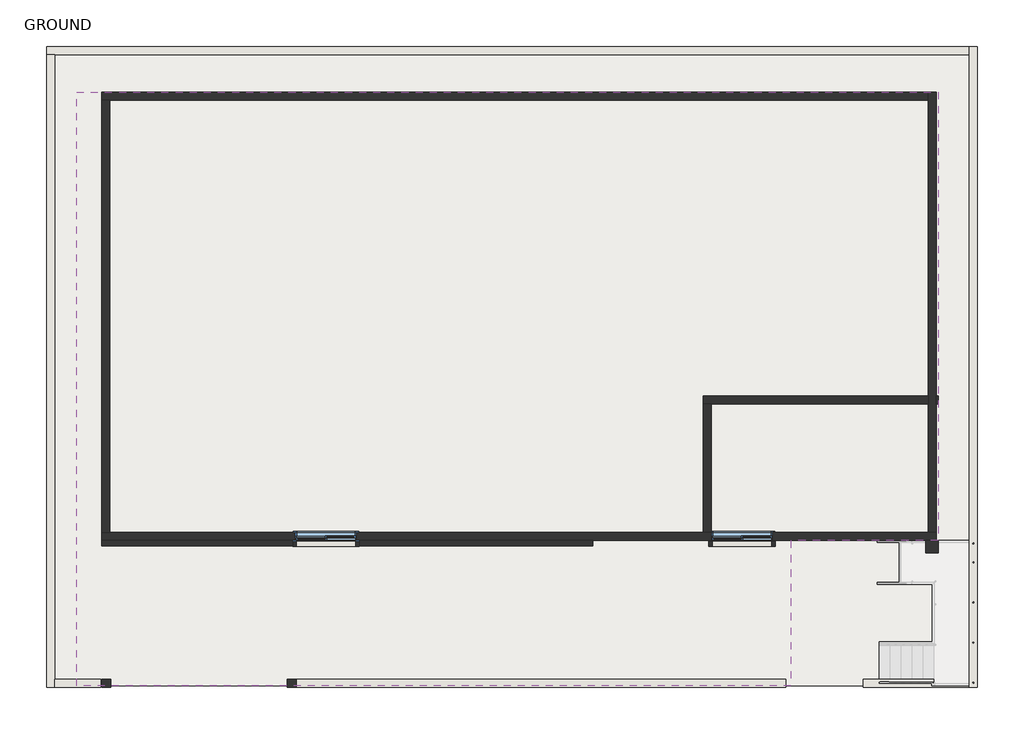
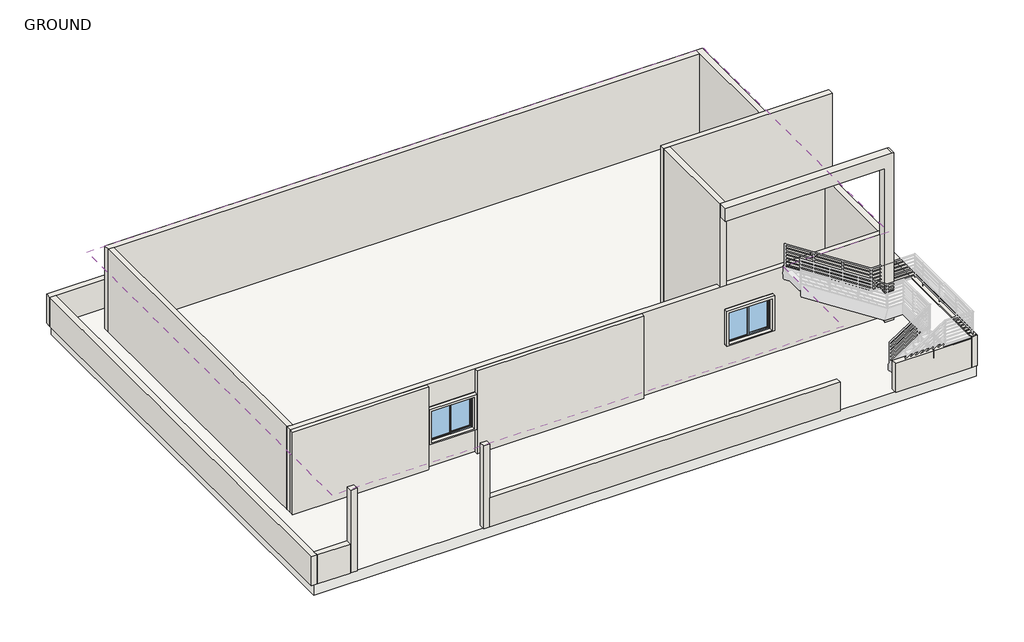
# One storey, part 1 of 4: 16 walls, 2 windows, 1 covering, 1 slab.
"""IFC4 building model written with IfcOpenShell, lengths in millimetres."""

from ifc_helpers import new_model, si_unit, frame, origin, origin_with_axes, place, context, project, spatial, polyline, outline, extrude, faceted_brep, transform, mapped, element, save
from components import walls_1_walls_1_df8d36ee, walls_2_walls_2_bd2c14ef, walls_3_walls_3_79010243, walls_4_walls_4_3dff52d5, window_c4d7a2b1

model = new_model("IFC4")

# Units and contexts
model_context = context("Model", 3, world=origin())
ifc_project = project(units=[si_unit("LENGTHUNIT", "METRE", prefix="MILLI")], contexts=[model_context])

# Site, building, storey
site = spatial("IfcSite", under=ifc_project)
building = spatial("IfcBuilding", under=site)
storey = spatial("IfcBuildingStorey", under=building, Name="GROUND", Elevation=0.0)

# Covering
placement = place(None, origin())
element("IfcCovering", 1, ObjectType="600 x 1200mm grid", at=placement, inside=storey, context=model_context, shape_type="SweptSolid", body=[
    extrude(outline(polyline([(-8160.4509113, 11210.9156744), (13293.8008502, 11210.9156744), (13293.8008502, 38.1156744), (9625.7864069, 38.1156744), (9625.7864069, -3583.7536983), (-8160.4509113, -3583.7536983), (-8160.4509113, 11210.9156744)])), frame((0.0, 0.0, 3048.0), z_axis=(0.0, 0.0, 1.0), x_axis=(1.0, 0.0, 0.0)), (0.0, 0.0, 1.0), 52.0),
])

# Slab
element("IfcSlab", 2, ObjectType="Generic Floor - 400mm", at=placement, inside=storey, context=model_context, shape_type="SweptSolid", body=[
    extrude(outline(polyline([(14250.8121881, 12248.1468238), (14250.8121881, -3583.7536983), (-8810.7878119, -3583.7536983), (-8810.7878119, 12248.1468238), (14250.8121881, 12248.1468238)])), frame((0.0, 0.0, -400.0), z_axis=(0.0, 0.0, 1.0), x_axis=(1.0, 0.0, 0.0)), (0.0, 0.0, 1.0), 400.0),
])

# Walls
element("IfcWall", 3, ObjectType="Generic - 9\"", at=placement, inside=storey, context=model_context, shape_type="Brep", body=[
    faceted_brep([(-7539.1878119, 11010.9156744, 0.0), (-7339.1878119, 11010.9156744, 0.0), (13053.0639497, 11010.9156744, 0.0), (13053.0639497, 11010.9156744, 3048.0), (-7339.1878119, 11010.9156744, 3048.0), (-7539.1878119, 11010.9156744, 3048.0), (-7539.1878119, 11210.9156744, 0.0), (-7539.1878119, 11210.9156744, 3048.0), (13053.0639497, 11210.9156744, 3048.0), (13053.0639497, 11210.9156744, 0.0)], [[[0, 1, 2, 3, 4, 5]], [[6, 7, 8, 9]], [[2, 1, 0, 6, 9]], [[5, 4, 3, 8, 7]], [[0, 5, 7, 6]], [[3, 2, 9, 8]]]),
])
element("IfcWall", 4, ObjectType="Generic - 9\"", at=placement, inside=storey, context=model_context, shape_type="SweptSolid", body=[
    extrude(outline(polyline([(-7339.1878119, 11010.9156744), (-7339.1878119, 238.1156744), (-7539.1878119, 238.1156744), (-7539.1878119, 11010.9156744), (-7339.1878119, 11010.9156744)])), origin_with_axes(), (0.0, 0.0, 1.0), 3048.0),
])
element("IfcWall", 5, ObjectType="Generic - 9\"", at=placement, inside=storey, context=model_context, shape_type="Brep", body=[
    faceted_brep([(13053.0639497, 11210.9156744, 0.0), (13053.0639497, 11010.9156744, 0.0), (13053.0639497, 3643.3156744, 0.0), (13053.0639497, 3443.3156744, 0.0), (13053.0639497, 238.1156744, 0.0), (13053.0639497, 238.1156744, 3048.0), (13053.0639497, 3443.3156744, 3048.0), (13053.0639497, 3643.3156744, 3048.0), (13053.0639497, 11010.9156744, 3048.0), (13053.0639497, 11210.9156744, 3048.0), (13253.0639497, 11210.9156744, 0.0), (13253.0639497, 11210.9156744, 3048.0), (13253.0639497, 3643.3156744, 3048.0), (13253.0639497, 3443.3156744, 3048.0), (13253.0639497, 238.1156744, 3048.0), (13253.0639497, 238.1156744, 0.0), (13253.0639497, 3443.3156744, 0.0), (13253.0639497, 3643.3156744, 0.0)], [[[0, 1, 2, 3, 4, 5, 6, 7, 8, 9]], [[10, 11, 12, 13, 14, 15, 16, 17]], [[4, 3, 2, 1, 0, 10, 17, 16, 15]], [[9, 8, 7, 6, 5, 14, 13, 12, 11]], [[0, 9, 11, 10]], [[5, 4, 15, 14]]]),
])
element("IfcWall", 6, ObjectType="Generic - 9\"", at=placement, inside=storey, context=model_context, shape_type="Brep", body=[
    faceted_brep([(-7539.1878119, 38.1156744, 0.0), (13253.0639497, 38.1156744, 0.0), (13253.0639497, 38.1156744, 3048.0), (-7539.1878119, 38.1156744, 3048.0), (-2714.7878119, 38.1156744, 2133.6), (-1190.7878119, 38.1156744, 2133.6), (-1190.7878119, 38.1156744, 914.4), (-2714.7878119, 38.1156744, 914.4), (7648.4121881, 38.1156744, 2133.6), (9172.4121881, 38.1156744, 2133.6), (9172.4121881, 38.1156744, 914.4), (7648.4121881, 38.1156744, 914.4), (-7539.1878119, 238.1156744, 0.0), (-7539.1878119, 238.1156744, 3048.0), (-7339.1878119, 238.1156744, 3048.0), (7439.6639497, 238.1156744, 3048.0), (7639.6639497, 238.1156744, 3048.0), (13053.0639497, 238.1156744, 3048.0), (13253.0639497, 238.1156744, 3048.0), (13253.0639497, 238.1156744, 0.0), (13053.0639497, 238.1156744, 0.0), (7639.6639497, 238.1156744, 0.0), (7439.6639497, 238.1156744, 0.0), (-7339.1878119, 238.1156744, 0.0), (-2714.7878119, 238.1156744, 2133.6), (-2714.7878119, 238.1156744, 914.4), (-1190.7878119, 238.1156744, 914.4), (-1190.7878119, 238.1156744, 2133.6), (7648.4121881, 238.1156744, 2133.6), (7648.4121881, 238.1156744, 914.4), (9172.4121881, 238.1156744, 914.4), (9172.4121881, 238.1156744, 2133.6)], [[[0, 1, 2, 3], [4, 5, 6, 7], [8, 9, 10, 11]], [[12, 13, 14, 15, 16, 17, 18, 19, 20, 21, 22, 23], [24, 25, 26, 27], [28, 29, 30, 31]], [[1, 0, 12, 23, 22, 21, 20, 19]], [[3, 2, 18, 17, 16, 15, 14, 13]], [[25, 24, 4, 7]], [[26, 25, 7, 6]], [[27, 26, 6, 5]], [[24, 27, 5, 4]], [[29, 28, 8, 11]], [[30, 29, 11, 10]], [[31, 30, 10, 9]], [[28, 31, 9, 8]], [[2, 1, 19, 18]], [[0, 3, 13, 12]]]),
])
element("IfcWall", 7, ObjectType="Generic - 9\"", at=placement, inside=storey, context=model_context, shape_type="Brep", body=[
    faceted_brep([(13293.8008502, 3443.3156744, 6096.0), (13093.8008502, 3443.3156744, 6096.0), (7639.6639497, 3443.3156744, 6096.0), (7439.6639497, 3443.3156744, 6096.0), (7439.6639497, 3443.3156744, 0.0), (7639.6639497, 3443.3156744, 0.0), (13053.0639497, 3443.3156744, 0.0), (13053.0639497, 3443.3156744, 3048.0), (13093.8008502, 3443.3156744, 3048.0), (13253.0639497, 3443.3156744, 3048.0), (13253.0639497, 3443.3156744, 0.0), (13293.8008502, 3443.3156744, 0.0), (13293.8008502, 3443.3156744, 3048.0), (7439.6639497, 3643.3156744, 6096.0), (13293.8008502, 3643.3156744, 6096.0), (13293.8008502, 3643.3156744, 0.0), (13253.0639497, 3643.3156744, 0.0), (13253.0639497, 3643.3156744, 3048.0), (13053.0639497, 3643.3156744, 3048.0), (13053.0639497, 3643.3156744, 0.0), (7439.6639497, 3643.3156744, 0.0)], [[[0, 1, 2, 3, 4, 5, 6, 7, 8, 9, 10, 11, 12]], [[13, 14, 15, 16, 17, 18, 19, 20]], [[4, 20, 19, 6, 5]], [[15, 11, 10, 16]], [[3, 2, 1, 0, 14, 13]], [[4, 3, 13, 20]], [[18, 7, 6, 19]], [[9, 17, 16, 10]], [[7, 18, 17, 9, 8]], [[0, 12, 11, 15, 14]]]),
])
element("IfcWall", 8, ObjectType="Generic - 9\"", at=placement, inside=storey, context=model_context, shape_type="Brep", body=[
    faceted_brep([(7639.6639497, 238.1156744, 0.0), (7639.6639497, 3443.3156744, 0.0), (7639.6639497, 3443.3156744, 6096.0), (7639.6639497, 238.1156744, 6096.0), (7639.6639497, 38.1156744, 6096.0), (7639.6639497, 38.1156744, 3048.0), (7639.6639497, 238.1156744, 3048.0), (7439.6639497, 238.1156744, 0.0), (7439.6639497, 238.1156744, 3048.0), (7439.6639497, 38.1156744, 3048.0), (7439.6639497, 38.1156744, 6096.0), (7439.6639497, 3443.3156744, 6096.0), (7439.6639497, 3443.3156744, 0.0)], [[[0, 1, 2, 3, 4, 5, 6]], [[7, 8, 9, 10, 11, 12]], [[1, 0, 7, 12]], [[4, 3, 2, 11, 10]], [[2, 1, 12, 11]], [[5, 9, 8, 6]], [[0, 6, 8, 7]], [[5, 4, 10, 9]]]),
])
element("IfcWall", 9, ObjectType="Generic - 9\"", at=placement, inside=storey, context=model_context, shape_type="Brep", body=[
    faceted_brep([(-8910.7878119, 12148.1468238, 0.0), (-8710.7878119, 12148.1468238, 0.0), (14075.4121881, 12148.1468238, 0.0), (14075.4121881, 12148.1468238, 1066.8), (-8710.7878119, 12148.1468238, 1066.8), (-8910.7878119, 12148.1468238, 1066.8), (-8910.7878119, 12348.1468238, 0.0), (-8910.7878119, 12348.1468238, 1066.8), (14075.4121881, 12348.1468238, 1066.8), (14075.4121881, 12348.1468238, 0.0)], [[[0, 1, 2, 3, 4, 5]], [[6, 7, 8, 9]], [[2, 1, 0, 6, 9]], [[5, 4, 3, 8, 7]], [[0, 5, 7, 6]], [[3, 2, 9, 8]]]),
])
element("IfcWall", 10, ObjectType="Generic - 9\"", at=placement, inside=storey, context=model_context, shape_type="Brep", body=[
    faceted_brep([(-8710.7878119, -3620.8536983, 0.0), (-8710.7878119, -3420.8536983, 0.0), (-8710.7878119, 12148.1468238, 0.0), (-8710.7878119, 12148.1468238, 1066.8), (-8710.7878119, -3420.8536983, 1066.8), (-8710.7878119, -3620.8536983, 1066.8), (-8910.7878119, -3620.8536983, 0.0), (-8910.7878119, -3620.8536983, 1066.8), (-8910.7878119, 12148.1468238, 1066.8), (-8910.7878119, 12148.1468238, 0.0)], [[[0, 1, 2, 3, 4, 5]], [[6, 7, 8, 9]], [[2, 1, 0, 6, 9]], [[5, 4, 3, 8, 7]], [[3, 2, 9, 8]], [[0, 5, 7, 6]]]),
])
element("IfcWall", 11, ObjectType="Generic - 9\"", at=placement, inside=storey, context=model_context, shape_type="Brep", body=[
    faceted_brep([(14075.4121881, 12348.1468238, 0.0), (14075.4121881, 12148.1468238, 0.0), (14075.4121881, -3420.8536983, 0.0), (14075.4121881, -3620.8536983, 0.0), (14075.4121881, -3620.8536983, 1066.8), (14075.4121881, -3620.8536983, 1123.1584328), (14075.4121881, 12348.1468238, 1123.1584328), (14075.4121881, 12348.1468238, 1066.8), (14275.4121881, 12348.1468238, 0.0), (14275.4121881, 12348.1468238, 1123.1584328), (14275.4121881, -3620.8536983, 1123.1584328), (14275.4121881, -3620.8536983, 0.0)], [[[0, 1, 2, 3, 4, 5, 6, 7]], [[8, 9, 10, 11]], [[3, 2, 1, 0, 8, 11]], [[6, 5, 10, 9]], [[0, 7, 6, 9, 8]], [[5, 4, 3, 11, 10]]]),
])
element("IfcWall", 12, ObjectType="Generic - 9\"", at=placement, inside=storey, context=model_context, shape_type="SweptSolid", body=[
    extrude(outline(polyline([(9496.2621881, -3620.8536983), (-2695.7378119, -3620.8536983), (-2695.7378119, -3420.8536983), (9496.2621881, -3420.8536983), (9496.2621881, -3620.8536983)])), origin_with_axes(), (0.0, 0.0, 1.0), 1066.8),
])
element("IfcWall", 13, ObjectType="Generic - 9\"", at=placement, inside=storey, context=model_context, shape_type="SweptSolid", body=[
    extrude(outline(polyline([(14075.4121881, -3620.8536983), (11432.2121881, -3620.8536983), (11432.2121881, -3420.8536983), (14075.4121881, -3420.8536983), (14075.4121881, -3620.8536983)])), origin_with_axes(), (0.0, 0.0, 1.0), 1066.8),
])
element("IfcWall", 14, ObjectType="Generic - 9\"", at=placement, inside=storey, context=model_context, shape_type="SweptSolid", body=[
    extrude(outline(polyline([(-7566.1878119, -3620.8536983), (-8710.7878119, -3620.8536983), (-8710.7878119, -3420.8536983), (-7566.1878119, -3420.8536983), (-7566.1878119, -3620.8536983)])), origin_with_axes(), (0.0, 0.0, 1.0), 1066.8),
])
walls_1_walls_1_shape = walls_1_walls_1_df8d36ee(model_context)
element("IfcWall", 15, ObjectType="Walls 1 : Walls 1", at=placement, inside=storey, context=model_context, shape_type="MappedRepresentation", body=[
    mapped(walls_1_walls_1_shape, transform((0.0, 0.0, 0.0), x_axis=(1.0, 0.0, 0.0), y_axis=(0.0, 1.0, 0.0), z_axis=(0.0, 0.0, 1.0))),
])
walls_2_walls_2_shape = walls_2_walls_2_bd2c14ef(model_context)
element("IfcWall", 16, ObjectType="Walls 2 : Walls 2", at=placement, inside=storey, context=model_context, shape_type="MappedRepresentation", body=[
    mapped(walls_2_walls_2_shape, transform((0.0, 0.0, 0.0), x_axis=(1.0, 0.0, 0.0), y_axis=(0.0, 1.0, 0.0), z_axis=(0.0, 0.0, 1.0))),
])
walls_3_walls_3_shape = walls_3_walls_3_79010243(model_context)
element("IfcWall", 17, ObjectType="Walls 3 : Walls 3", at=placement, inside=storey, context=model_context, shape_type="MappedRepresentation", body=[
    mapped(walls_3_walls_3_shape, transform((0.0, 0.0, 0.0), x_axis=(1.0, 0.0, 0.0), y_axis=(0.0, 1.0, 0.0), z_axis=(0.0, 0.0, 1.0))),
])
walls_4_walls_4_shape = walls_4_walls_4_3dff52d5(model_context)
element("IfcWall", 18, ObjectType="Walls 4 : Walls 4", at=placement, inside=storey, context=model_context, shape_type="MappedRepresentation", body=[
    mapped(walls_4_walls_4_shape, transform((0.0, 0.0, 0.0), x_axis=(1.0, 0.0, 0.0), y_axis=(0.0, 1.0, 0.0), z_axis=(0.0, 0.0, 1.0))),
])

# Windows
window_shape = window_c4d7a2b1(model_context)
element("IfcWindow", 19, ObjectType="Slider with Trim : 60\" x 48\"", at=placement, inside=storey, context=model_context, shape_type="MappedRepresentation", body=[
    mapped(window_shape, transform((-1952.7878119, 138.1156744, 0.0), x_axis=(-1.0, 0.0, 0.0), y_axis=(0.0, -1.0, 0.0), z_axis=(0.0, 0.0, 1.0))),
])
element("IfcWindow", 20, ObjectType="Slider with Trim : 60\" x 48\"", at=placement, inside=storey, context=model_context, shape_type="MappedRepresentation", body=[
    mapped(window_shape, transform((8410.4121881, 138.1156744, 0.0), x_axis=(-1.0, 0.0, 0.0), y_axis=(0.0, -1.0, 0.0), z_axis=(0.0, 0.0, 1.0))),
])

save(model, "model.ifc")

# Revit data of these elements
# Type "600 x 1200mm grid"
#   built-in parameter 1002203 = 1 (stored number, unit not read)
#   built-in parameter 1002202 = 1 (stored number, unit not read)
#   Layers, outside or top first: 0' - 1.41732" "Default" (function 1); 0' - 0.62992" "Ceiling Tile 600 x 1200" (function 5)
# Type "Generic Floor - 400mm"
#   Function = 0
#   Layers, outside or top first: 1' - 3.74803" no material (function 1)
# Type "Generic - 9\""
#   Layers, outside or top first: 0' - 7.87402" no material (function 1)
# Type "Slider with Trim : 60\" x 48\""
#   Type Mark = "22"
#   Construction Type Id = "GSP4R"
#   Assembly Code = "B2020100"
#   Analytic Construction = "1/8 in Pilkington single glazing"
#   Visual Light Transmittance = 0.9
#   Solar Heat Gain Coefficient = 0.78
#   Heat Transfer Coefficient (U) = 3.6886 W/(m²·K)
#   Height = 4' - 0"
#   Default Sill Height = 3' - 0"
#   Trim Projection - Ext. = 0' - 0 3/4"
#   Trim Projection - Int. = 0' - 0 3/4"
#   Trim Width - Exterior = 0' - 3 1/2"
#   Trim Width - Interior = 0' - 3 1/2"
#   Width = 5' - 0"
#   Window Inset = 0' - 0 3/4"
#   Define Thermal Properties by = 1
#   Glass Pane Material = Glass
#   Sash Material = Sash
#   Trim Exterior Material = Trim
#   Trim Interior Material = Trim
#   Wall Closure = (empty or 0)
# Element 1 (IfcCovering, "600 x 1200mm grid")
#   Height Offset From Level = 10' - 0"
#   Phase Created = New Construction
#   Materials on its faces: "Ceiling Tile 600 x 1200", "Default"
# Element 2 (IfcSlab, "Generic Floor - 400mm")
#   Height Offset From Level = 0' - 0"
#   Phase Created = New Construction
#   Materials on its faces: "Default Roof"
# Elements 3, 4, 5, 6 (IfcWall, "Generic - 9\"")
#   Top Offset = 0' - 0"
#   Base Offset = 0' - 0"
#   Unconnected Height = 10' - 0"
#   wall height = 10' - 0"
#   Phase Created = New Construction
#   Base Constraint = GROUND
#   Materials on its faces: "Default Wall"
# Elements 7, 8 (IfcWall, "Generic - 9\"")
#   Top Offset = 0' - 0"
#   Base Offset = 0' - 0"
#   Unconnected Height = 20' - 0"
#   wall height = 20' - 0"
#   Phase Created = New Construction
#   Base Constraint = GROUND
#   Materials on its faces: "Default Wall"
# Elements 9, 10, 12, 13, 14 (IfcWall, "Generic - 9\"")
#   Top Offset = 0' - 0"
#   Base Offset = 0' - 0"
#   Unconnected Height = 3' - 6"
#   wall height = 3' - 6"
#   Phase Created = New Construction
#   Base Constraint = GROUND
#   Materials on its faces: "Default Wall"
# Element 11 (IfcWall, "Generic - 9\"")
#   Top Offset = 0' - 0"
#   Base Offset = 0' - 0"
#   Unconnected Height = 3' - 8.21884"
#   wall height = 3' - 8.21884"
#   Phase Created = New Construction
#   Base Constraint = GROUND
#   Materials on its faces: "Default Wall"
# Element 15 (IfcWall, "Walls 1 : Walls 1")
#   Phase Created = New Construction
#   Materials on its faces: "Default Wall"
# Element 16 (IfcWall, "Walls 2 : Walls 2")
#   Phase Created = New Construction
#   Materials on its faces: "Default Wall"
# Element 17 (IfcWall, "Walls 3 : Walls 3")
#   Phase Created = New Construction
#   Materials on its faces: "Default Wall"
# Element 18 (IfcWall, "Walls 4 : Walls 4")
#   Phase Created = New Construction
#   Materials on its faces: "Default Wall"
# Element 19 (IfcWindow, "Slider with Trim : 60\" x 48\"")
#   Mark = "10"
#   Phase Created = New Construction
#   Materials on its faces: "Sash", "Trim", "Glass"
# Element 20 (IfcWindow, "Slider with Trim : 60\" x 48\"")
#   Mark = "11"
#   Phase Created = New Construction
#   Materials on its faces: "Sash", "Trim", "Glass"
# Materials
#   "Default": colour RGB 80 80 80, transparency 0
#   "Ceiling Tile 600 x 1200": class "Generic", colour RGB 179 178 175, transparency 0, Description = "Acoustic ceiling tile", Cost = 0
#   "Glass": class "Glass", colour RGB 218 227 224, transparency 0.85, Description = "Soda Lime Glass", Cost = 0
#   "Sash": class "Wood", colour RGB 136 99 55, transparency 0
#   "Trim": class "Wood", colour RGB 224 178 126, transparency 0
#   "Default Roof": colour RGB 80 80 80, transparency 0
#   "Default Wall": colour RGB 80 80 80, transparency 0
